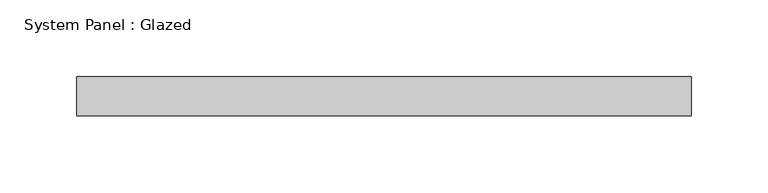
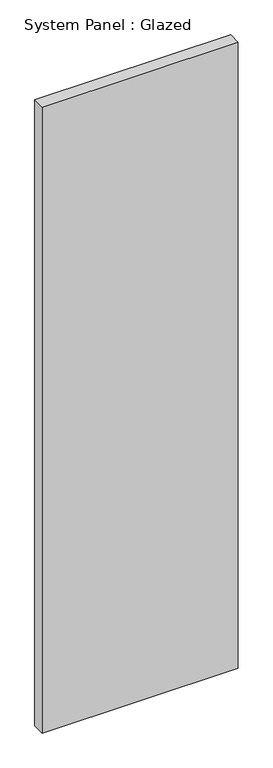
"""IFC4 building model written with IfcOpenShell, lengths in millimetres: plate geometry, System Panel : Glazed."""

from ifc_helpers import new_model, si_unit, origin, origin_with_axes, place, context, project, spatial, polyline, outline, extrude, source, transform, mapped, element, save


def system_panel_glazed_32fc5117(model_context):
    return source(origin(), model_context, "Body", "SweptSolid", [
        extrude(outline(polyline([(200.025, 19.05), (-200.025, 19.05), (-200.025, 44.45), (200.025, 44.45), (200.025, 19.05)])), origin_with_axes(), (0.0, 0.0, 1.0), 1348.7821201),
    ])


if __name__ == "__main__":
    model = new_model("IFC4")
    model_context = context("Model", 3, world=origin())
    ifc_project = project(units=[si_unit("LENGTHUNIT", "METRE", prefix="MILLI")], contexts=[model_context])
    site = spatial("IfcSite", under=ifc_project)
    building = spatial("IfcBuilding", under=site)
    placement = place(None, origin())
    system_panel_glazed_shape = system_panel_glazed_32fc5117(model_context)
    element("IfcPlate", 1, ObjectType="System Panel : Glazed", at=placement, inside=building, context=model_context, shape_type="MappedRepresentation", body=[
        mapped(system_panel_glazed_shape, transform((0.0, 0.0, 0.0), x_axis=(1.0, 0.0, 0.0), y_axis=(0.0, 1.0, 0.0), z_axis=(0.0, 0.0, 1.0))),
    ])
    save(model, "model.ifc")

# Revit data of these elements
# Type "System Panel : Glazed"
#   Construction Type Id = "GSP4R"
#   Analytic Construction = "1/8 in Pilkington single glazing"
#   Visual Light Transmittance = 0.9
#   Solar Heat Gain Coefficient = 0.86
#   Heat Transfer Coefficient (U) = 1.18115 BTU/(h·ft²·°F)
#   Define Thermal Properties by = 1
# Element 1 (IfcPlate, "System Panel : Glazed")
#   Materials on its faces: "Glass"
# Materials
#   "Glass": class "Glass", colour RGB 0 128 192, transparency 0.75, Description = "Soda Lime Glass", Cost = 0
